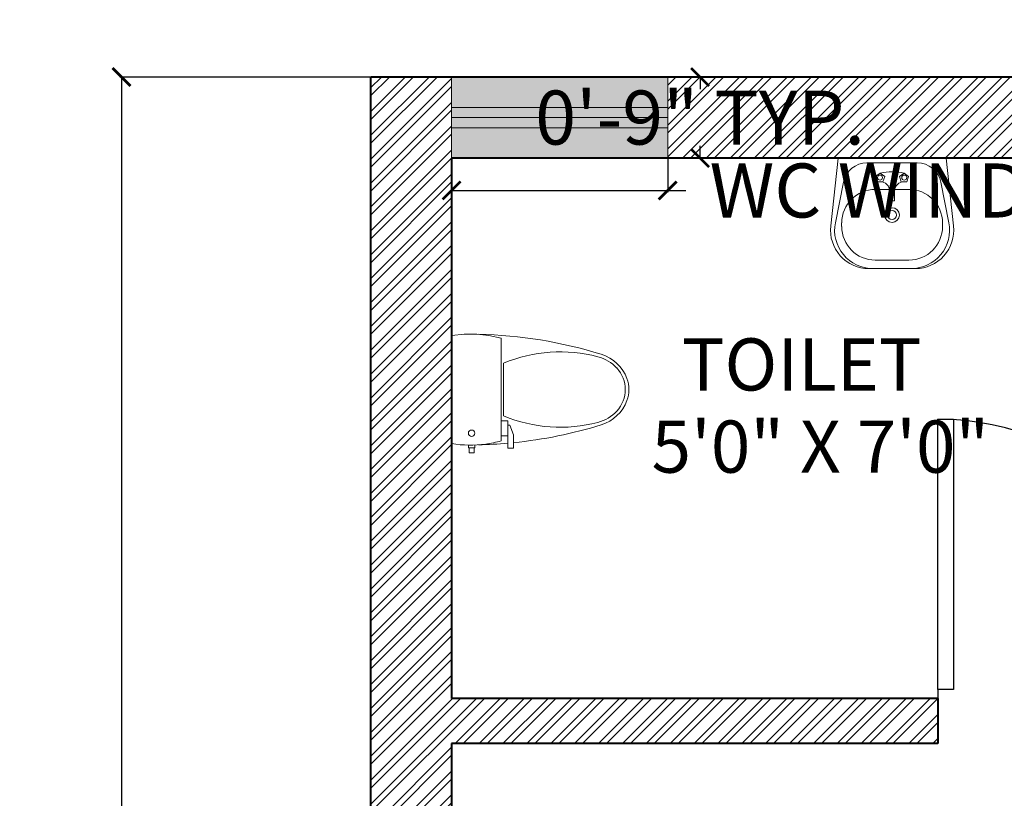
# Model space of a CAD drawing. Units: inches. Extents: x 528 to 2520, y -151 to 1354.
# Tile 34 of 41: x 2119 to 2228, y 818 to 904. Entities that reach past the tile are written whole.
import ezdxf

# ---------------------------------------------------------------- set-up
doc = ezdxf.new("R2010")
doc.units = ezdxf.units.IN
doc.header["$MEASUREMENT"] = 0
for name, color, linetype, lineweight in [('A-ANNO-DIMS', 2, 'Continuous', 18), ('A-AREA-IDEN', 7, 'Continuous', 18), ('A-Door', 150, 'Continuous', 25), ('A-ELEV-PROJ', 8, 'Continuous', 13), ('A-FLOR-FIXT', 9, 'Continuous', 18), ('A-WALL-PATT', 6, 'Continuous', 13), ('walls', 7, 'Continuous', 40), ('WINDOWS', 2, 'Continuous', 20)]:
    doc.layers.add(name, color=color, linetype=linetype, lineweight=lineweight)
doc.layers.add('A-GLAZ-PATT', color=152, linetype='Continuous', lineweight=13, true_color=0x2776bb)
doc.styles.get("Standard").update_dxf_attribs({"font": 'arial.ttf'})
doc.dimstyles.get("Standard").update_dxf_attribs({"dimtxt": 6, "dimasz": 2, "dimexe": 0.18, "dimexo": 0.0625, "dimgap": 0.09, "dimtad": 0, "dimtih": 1, "dimtoh": 1, "dimdec": 1, "dimzin": 0, "dimdsep": 46, "dimlunit": 3, "dimtxsty": 'Standard', "dimblk": 'ARCHTICK', "dimcen": 0.09, "dimadec": 0, "dimazin": 0, "dimtfac": 1, "dimtdec": 1, "dimtofl": 0, "dimtmove": 0, "dimatfit": 3, "dimfxl": 1, "dimtolj": 1, "dimtzin": 0, "dimarcsym": 0})

# ---------------------------------------------------------------- blocks, each defined once
blk = doc.blocks.new('toilet-7')
at = {"color": 0, "linetype": 'ByBlock'}
for p, q in [((0.2097, -0.02), (-0.2097, -0.02)), ((0.2151, -0.0677), (0.2097, -0.02)), ((0.2151, -0.1171), (0.2151, -0.0677)), ((-0.2457, -0.0874), (-0.2457, -0.1068)), ((-0.2457, -0.0874), (-0.2257, -0.0874)), ((-0.2457, -0.1068), (-0.2257, -0.1068)), ((-0.2257, -0.0846), (-0.2257, -0.1096)), ((-0.2257, -0.0846), (-0.2157, -0.0846)), ((-0.2257, -0.1096), (-0.2154, -0.1096)), ((0.2099, -0.164), (0.2151, -0.1171)), ((0.1991, -0.2124), (0.2099, -0.164)), ((0.1991, -0.2124), (-0.1991, -0.2124)), ((-0.1803, -0.2374), (-0.1803, -0.2124)), ((-0.1213, -0.2374), (-0.1213, -0.2124)), ((-0.1023, -0.2212), (0.1023, -0.2212)), ((-0.1213, -0.2374), (-0.2278, -0.2374)), ((-0.2278, -0.2374), (-0.2278, -0.2599)), ((-0.1759, -0.2599), (-0.2278, -0.2599)), ((-0.1759, -0.2599), (-0.1379, -0.2451)), ((-0.1379, -0.2451), (-0.1379, -0.2374))]:
    blk.add_line(p, q, dxfattribs=at)
blk.add_circle((-0.1696, -0.0971), 0.0125, dxfattribs=at)
for centre, radius, start, end in [((0.2244, -0.0924), 0.4402, 170.5377, 187.7399), ((1.517, -0.087), 1.7318, 181.2224, 184.9822), ((0.2244, -0.0924), 0.4402, 187.7399, 195.822), ((-1.517, -0.087), 1.7318, 342.7523, 358.7776), ((0.4258, -0.4413), 0.5721, 157.3737, 194.7786), ((-0.4258, -0.4413), 0.5721, 345.2214, 22.6263), ((1.517, -0.087), 1.7318, 185.7323, 197.2477), ((0.0116, -0.5544), 0.1554, 197.2477, 249.5476), ((0.0221, -0.5478), 0.1546, 194.7786, 226.8543), ((-0.0116, -0.5544), 0.1554, 290.4524, 342.7523), ((-0.0221, -0.5478), 0.1546, 313.1457, 345.2214), ((0, -0.5713), 0.1223, 226.8543, 313.1457), ((0, -0.5854), 0.1223, 249.5476, 290.4524)]:
    blk.add_arc(centre, radius, start, end, dxfattribs=at)
blk = doc.blocks.new('BASIN-WITH-TAP')
for p, q in [((0.84, 12.27), (0.02, 4.73)), ((12.84, 12.27), (0.84, 12.27)), ((12.84, 12.27), (13.66, 4.73)), ((9.64, 11.73), (4.05, 11.73)), ((5, 10.24), (5.51, 10.61)), ((5.2, 9.64), (5, 10.24)), ((5.24, 10.1), (5.2, 10.1)), ((5.51, 10.61), (6.02, 10.24)), ((6.02, 10.24), (5.82, 9.64)), ((8.18, 10.61), (7.67, 10.24)), ((7.67, 10.24), (7.86, 9.64)), ((8.68, 10.24), (8.18, 10.61)), ((8.44, 10.1), (8.49, 10.1)), ((8.49, 9.64), (8.68, 10.24)), ((1.43, 9.58), (0.55, 5.09)), ((4.98, 8.8), (6.58, 8.8)), ((5.24, 9.64), (5.51, 9.64)), ((8.71, 8.8), (7.11, 8.8)), ((8.49, 9.64), (8.18, 9.64)), ((12.26, 9.58), (13.14, 5.09)), ((6.58, 8.31), (6.58, 8.58)), ((6.58, 7.51), (6.58, 8.31)), ((7.11, 8.31), (7.11, 8.58)), ((7.11, 7.51), (7.11, 8.31)), ((6.58, 7.51), (7.11, 7.51)), ((1.24, 4.67), (1.24, 5.07)), ((12.44, 4.67), (12.44, 5.07)), ((4.73, 0), (8.96, 0)), ((6.84, 0.93), (4.98, 0.93)), ((6.84, 0.93), (8.71, 0.93))]:
    blk.add_line(p, q)
for centre, radius in [((5.5, 10.1), 0.277), ((8.19, 10.1), 0.277), ((6.84, 5.94), 0.821), ((6.84, 5.94), 0.507)]:
    blk.add_circle(centre, radius)
for centre, radius, start, end in [((4.05, 9.07), 2.67, 90, 168.8773), ((9.64, 9.07), 2.67, 11.1227, 90), ((6.84, 4.01), 6.73, 78.5788, 101.4212), ((4.98, 5.07), 3.73, 90, 180), ((5.51, 8.58), 1.07, 0, 90), ((8.18, 8.58), 1.07, 90, 180), ((8.71, 5.07), 3.73, 0, 90), ((4.27, 4.27), 4.27, 173.7966, 270), ((4.73, 4.27), 4.27, 168.8773, 270), ((4.98, 4.67), 3.73, 180, 270), ((8.71, 4.67), 3.73, 270, 0), ((8.96, 4.27), 4.27, 270, 11.1227), ((9.42, 4.27), 4.27, 270, 6.2034)]:
    blk.add_arc(centre, radius, start, end)
blk = doc.blocks.new('DOOR-SWING-30')
for p, q in [((0, 6), (0, 0)), ((30, 6), (30, 0))]:
    blk.add_line(p, q)
blk.add_lwpolyline([(0, 6), (0, 36), (1.75, 36), (1.75, 6)], close=True)
blk.add_arc((0, 6), 30, 0, 90)
blk = doc.blocks.new('WINDOW-24x9-PLAN')
for p, q in [((0, 5.63), (24, 5.63)), ((0, 4.5), (24, 4.5)), ((0, 3.37), (24, 3.37))]:
    blk.add_line(p, q)
blk.add_lwpolyline([(0, 9), (24, 9), (24, 0), (0, 0)], close=True)
blk = doc.blocks.new('_ArchTick')
at = {"color": 0, "linetype": 'ByBlock', "const_width": 0.15}
blk.add_lwpolyline([(-0.5, -0.5), (0.5, 0.5)], dxfattribs=at)
blk = doc.blocks.new('*D56')
at = {"layer": 'A-ANNO-DIMS', "color": 0, "lineweight": -2, "transparency": 16777216}
for p, q in [((2167.01, 888.88), (2167.01, 885.16)), ((2191.01, 888.88), (2191.01, 885.16)), ((2167.01, 885.34), (2191.01, 885.34)), ((2191.01, 885.34), (2193.01, 885.34))]:
    blk.add_line(p, q, dxfattribs=at)
at = {"layer": 'Defpoints', "color": 0, "transparency": 16777216}
for p in [(2167.01, 888.94), (2191.01, 888.94), (2191.01, 885.34)]:
    blk.add_point(p, dxfattribs=at)
at = {"layer": 'A-ANNO-DIMS', "color": 0, "lineweight": -2, "transparency": 16777216, "xscale": 2, "yscale": 2, "zscale": 2, "rotation": 180}
blk.add_blockref('_ArchTick', (2167.01, 885.34), dxfattribs=at)
at = {"layer": 'A-ANNO-DIMS', "color": 0, "lineweight": -2, "transparency": 16777216, "xscale": 2, "yscale": 2, "zscale": 2}
blk.add_blockref('_ArchTick', (2191.01, 885.34), dxfattribs=at)
at = {"layer": 'A-ANNO-DIMS', "color": 0, "transparency": 16777216, "insert": (2239.21, 885.34), "char_height": 6, "attachment_point": 5}
blk.add_mtext('\\A1;WC WINDOW 2\'-0" TYP.', dxfattribs=at)
blk = doc.blocks.new('*D57')
at = {"layer": 'A-ANNO-DIMS', "color": 0, "lineweight": -2, "transparency": 16777216}
for p, q in [((2191.07, 897.94), (2194.79, 897.94)), ((2194.61, 897.94), (2194.61, 896.59)), ((2194.61, 888.94), (2194.61, 890.29)), ((2191.07, 888.94), (2194.79, 888.94))]:
    blk.add_line(p, q, dxfattribs=at)
at = {"layer": 'Defpoints', "color": 0, "transparency": 16777216}
for p in [(2191.01, 897.94), (2194.61, 897.94), (2191.01, 888.94)]:
    blk.add_point(p, dxfattribs=at)
at = {"layer": 'A-ANNO-DIMS', "color": 0, "lineweight": -2, "transparency": 16777216, "xscale": 2, "yscale": 2, "zscale": 2}
for p, rotation in [((2194.61, 897.94), 90), ((2194.61, 888.94), 270)]:
    blk.add_blockref('_ArchTick', p, dxfattribs=dict(at, rotation=rotation))
at = {"layer": 'A-ANNO-DIMS', "color": 0, "transparency": 16777216, "insert": (2194.61, 893.44), "char_height": 6, "attachment_point": 5}
blk.add_mtext('\\A1;0\'-9" TYP.', dxfattribs=at)
blk = doc.blocks.new('*D95')
at = {"layer": 'A-ANNO-DIMS', "color": 0, "lineweight": -2, "transparency": 16777216}
for p, q in [((2157.95, 897.94), (2130.18, 897.94)), ((2130.36, 897.94), (2130.36, 632.59)), ((2130.36, 360.94), (2130.36, 626.29)), ((2157.95, 360.94), (2130.18, 360.94))]:
    blk.add_line(p, q, dxfattribs=at)
at = {"layer": 'Defpoints', "color": 0, "transparency": 16777216}
for p in [(2130.36, 897.94), (2158.01, 897.94), (2158.01, 360.94)]:
    blk.add_point(p, dxfattribs=at)
at = {"layer": 'A-ANNO-DIMS', "color": 0, "lineweight": -2, "transparency": 16777216, "xscale": 2, "yscale": 2, "zscale": 2}
for p, rotation in [((2130.36, 897.94), 90), ((2130.36, 360.94), 270)]:
    blk.add_blockref('_ArchTick', p, dxfattribs=dict(at, rotation=rotation))
at = {"layer": 'A-ANNO-DIMS', "color": 0, "transparency": 16777216, "insert": (2130.36, 629.44), "char_height": 6, "attachment_point": 5}
blk.add_mtext('\\A1;44\'-9"', dxfattribs=at)

msp = doc.modelspace()

# ---------------------------------------------------------------- hatches: boundary and pattern name
at = {"layer": 'A-GLAZ-PATT'}
h = msp.add_hatch(color=256, dxfattribs=at)
h.dxf.hatch_style = 1
h.paths.add_polyline_path([(2191.01, 894.57), (2167.01, 894.57), (2167.01, 893.44), (2191.01, 893.44)])
h.paths.add_polyline_path([(2191.01, 893.44), (2167.01, 893.44), (2167.01, 892.31), (2191.01, 892.31)])
h.paths.add_polyline_path([(2191.01, 897.94), (2167.01, 897.94), (2167.01, 894.57), (2191.01, 894.57)])
h.paths.add_polyline_path([(2191.01, 892.31), (2167.01, 892.31), (2167.01, 888.94), (2191.01, 888.94)])
at = {"layer": 'A-WALL-PATT'}
h = msp.add_hatch(dxfattribs=at)
h.set_pattern_fill('ANSI32', color=256, scale=5)
h.set_pattern_definition([(45, (1571.3155, -419.1643), (-1.3258252, 1.3258252), []), (45, (1572.1993, -419.1643), (-1.3258252, 1.3258252), [])])
h.paths.add_polyline_path([(2167.01, 744.69), (2158.01, 744.69), (2158.01, 549.94), (2169.56, 549.94), (2174.56, 549.94), (2174.56, 554.94), (2167.01, 554.94), (2167.01, 662.94), (2263.01, 662.94), (2263.01, 667.94), (2263.01, 686.94), (2269.01, 686.94), (2269.01, 691.94), (2258.01, 691.94), (2258.01, 667.94), (2167.01, 667.94)])
h.paths.add_polyline_path([(2260.02, 554.94), (2222.56, 554.94), (2222.56, 549.94), (2260.02, 549.94)])
h.paths.add_polyline_path([(2457.01, 752.2), (2448.01, 752.2), (2448.01, 691.94), (2358.01, 691.94), (2358.01, 686.94), (2448.01, 686.94), (2448.01, 554.94), (2358.01, 554.94), (2358.01, 549.94), (2448.01, 549.94), (2448.01, 405.94), (2406.01, 405.94), (2406.01, 396.94), (2457.01, 396.94)])
h.paths.add_polyline_path([(2457.01, 897.94), (2447.97, 897.94), (2447.97, 888.94), (2448.01, 888.94), (2448.01, 828.94), (2394.01, 828.94), (2394.01, 823.94), (2448.01, 823.94), (2448.01, 800.2), (2457.01, 800.2)])
h.paths.add_polyline_path([(2423.97, 897.94), (2359.01, 897.94), (2359.01, 828.94), (2355.58, 828.94), (2355.58, 823.94), (2364.01, 823.94), (2364.01, 829.94), (2364.01, 888.94), (2423.97, 888.94)])
h.paths.add_polyline_path([(2256.01, 897.94), (2191.01, 897.94), (2191.01, 888.94), (2251.01, 888.94), (2251.01, 828.94), (2251.01, 823.94), (2256.01, 823.94), (2256.01, 829.08)])
h.paths.add_polyline_path([(2167.01, 888.94), (2167.01, 897.94), (2158.01, 897.94), (2158.01, 792.69), (2167.01, 792.69), (2167.01, 823.94), (2221.01, 823.94), (2221.01, 828.94), (2167.01, 828.94)])
h.paths.add_polyline_path([(2316.01, 549.94), (2316.01, 554.94), (2296.02, 554.94), (2296.02, 549.94), (2311.01, 549.94), (2311.01, 455.12), (2316.01, 455.12)])
h.paths.add_polyline_path([(2311.01, 549.94), (2299.01, 549.94), (2299.01, 545.95), (2302.05, 545.95), (2302.05, 542.51), (2305.75, 542.51), (2305.75, 538.08), (2311.01, 538.08)], flags=17)
h.paths.add_polyline_path([(2358.01, 405.94), (2316.01, 405.94), (2316.01, 413.12), (2311.01, 413.12), (2311.01, 396.94), (2358.01, 396.94)])

# ---------------------------------------------------------------- linework, layer by layer
at = {"layer": 'A-ELEV-PROJ'}
msp.add_line((2158.01, 360.94), (2158.01, 897.94), dxfattribs=at)
at = {"layer": 'walls'}
for p, q in [((2158.01, 897.94), (2158.01, 369.94)), ((2256.01, 897.94), (2158.01, 897.94)), ((2167.01, 888.94), (2167.01, 828.94)), ((2251.01, 888.94), (2167.01, 888.94)), ((2221.01, 828.94), (2167.01, 828.94)), ((2221.01, 828.94), (2221.01, 823.94)), ((2167.01, 823.94), (2167.01, 667.94)), ((2221.01, 823.94), (2167.01, 823.94))]:
    msp.add_line(p, q, dxfattribs=at)

# ---------------------------------------------------------------- block references
at = {"layer": 'A-Door'}
msp.add_blockref('DOOR-SWING-30', (2221.01, 823.94), dxfattribs=at)
at = {"layer": 'A-FLOR-FIXT'}
msp.add_blockref('BASIN-WITH-TAP', (2209.09, 876.67), dxfattribs=at)
at = {"layer": 'A-FLOR-FIXT', "xscale": 28.60654769571749, "yscale": 28.60654769571749, "zscale": 28.60654769571749, "rotation": 90}
msp.add_blockref('toilet-7', (2166.46, 863.24), dxfattribs=at)
at = {"layer": 'WINDOWS'}
msp.add_blockref('WINDOW-24x9-PLAN', (2167.01, 888.94), dxfattribs=at)

# ---------------------------------------------------------------- texts
at = {"layer": 'A-AREA-IDEN'}
for s, height, p in [('TOILET', 5.793, (2192.59, 863.13)), ('5\'0" X 7\'0"', 5.7926, (2189.22, 854.01))]:
    msp.add_text(s, height=height, dxfattribs=at).set_placement(p)

# ---------------------------------------------------------------- dimensions: what is measured, and where the dimension line sits
at = {"layer": 'A-ANNO-DIMS'}
dim = msp.add_linear_dim(base=(2191.01, 885.34), p1=(2167.01, 888.94), p2=(2191.01, 888.94), text='WC WINDOW <> TYP.', dimstyle='Standard', override={"dimdec": 1, "dimlfac": 1, "dimrnd": 0, "dimzin": 1, "dimdsep": 46, "dimlunit": 4, "dimfrac": 2}, dxfattribs=at)
dim.commit()
dim.dimension.update_dxf_attribs({"geometry": '*D56', "text_midpoint": (2239.21, 885.34)})
dim = msp.add_linear_dim(base=(2194.61, 897.94), p1=(2191.01, 888.94), p2=(2191.01, 897.94), angle=90, text='<> TYP.', dimstyle='Standard', override={"dimdec": 1, "dimlfac": 1, "dimrnd": 0, "dimzin": 1, "dimdsep": 46, "dimlunit": 4, "dimfrac": 2}, dxfattribs=at)
dim.commit()
dim.dimension.update_dxf_attribs({"geometry": '*D57', "text_midpoint": (2194.61, 893.44)})
dim = msp.add_linear_dim(base=(2130.36, 897.94), p1=(2158.01, 360.94), p2=(2158.01, 897.94), angle=90, dimstyle='Standard', override={"dimdec": 1, "dimlfac": 1, "dimrnd": 0, "dimzin": 1, "dimdsep": 46, "dimlunit": 4, "dimfrac": 2}, dxfattribs=at)
dim.commit()
dim.dimension.update_dxf_attribs({"geometry": '*D95', "text_midpoint": (2130.36, 629.44)})

doc.saveas('drawing.dxf')
